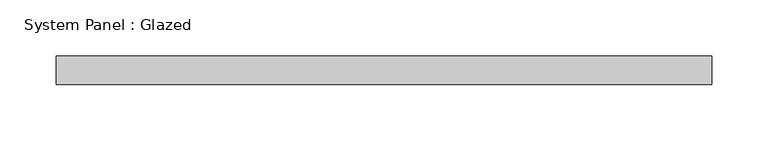
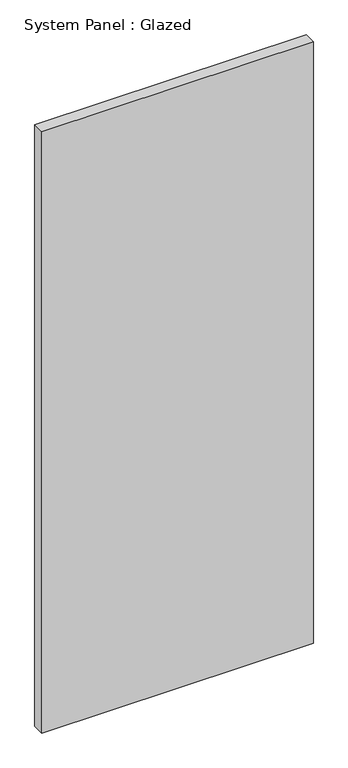
"""IFC4 building model written with IfcOpenShell, lengths in millimetres: plate geometry, System Panel : Glazed."""

from ifc_helpers import new_model, si_unit, origin, origin_with_axes, place, context, project, spatial, polyline, outline, extrude, source, transform, mapped, element, save


def system_panel_glazed_18fdb1ad(model_context):
    return source(origin(), model_context, "Body", "SweptSolid", [
        extrude(outline(polyline([(292.1, 19.05), (-292.1, 19.05), (-292.1, 44.45), (292.1, 44.45), (292.1, 19.05)])), origin_with_axes(), (0.0, 0.0, 1.0), 1366.5474484),
    ])


if __name__ == "__main__":
    model = new_model("IFC4")
    model_context = context("Model", 3, world=origin())
    ifc_project = project(units=[si_unit("LENGTHUNIT", "METRE", prefix="MILLI")], contexts=[model_context])
    site = spatial("IfcSite", under=ifc_project)
    building = spatial("IfcBuilding", under=site)
    placement = place(None, origin())
    system_panel_glazed_shape = system_panel_glazed_18fdb1ad(model_context)
    element("IfcPlate", 1, ObjectType="System Panel : Glazed", at=placement, inside=building, context=model_context, shape_type="MappedRepresentation", body=[
        mapped(system_panel_glazed_shape, transform((0.0, 0.0, 0.0), x_axis=(1.0, 0.0, 0.0), y_axis=(0.0, 1.0, 0.0), z_axis=(0.0, 0.0, 1.0))),
    ])
    save(model, "model.ifc")

# Revit data of these elements
# Type "System Panel : Glazed"
#   Construction Type Id = "GSP4R"
#   Analytic Construction = "1/8 in Pilkington single glazing"
#   Visual Light Transmittance = 0.9
#   Solar Heat Gain Coefficient = 0.86
#   Heat Transfer Coefficient (U) = 1.18115 BTU/(h·ft²·°F)
#   Define Thermal Properties by = 1
# Element 1 (IfcPlate, "System Panel : Glazed")
#   Materials on its faces: "Glass"
# Materials
#   "Glass": class "Glass", colour RGB 0 128 192, transparency 0.75, Description = "Soda Lime Glass", Cost = 0
